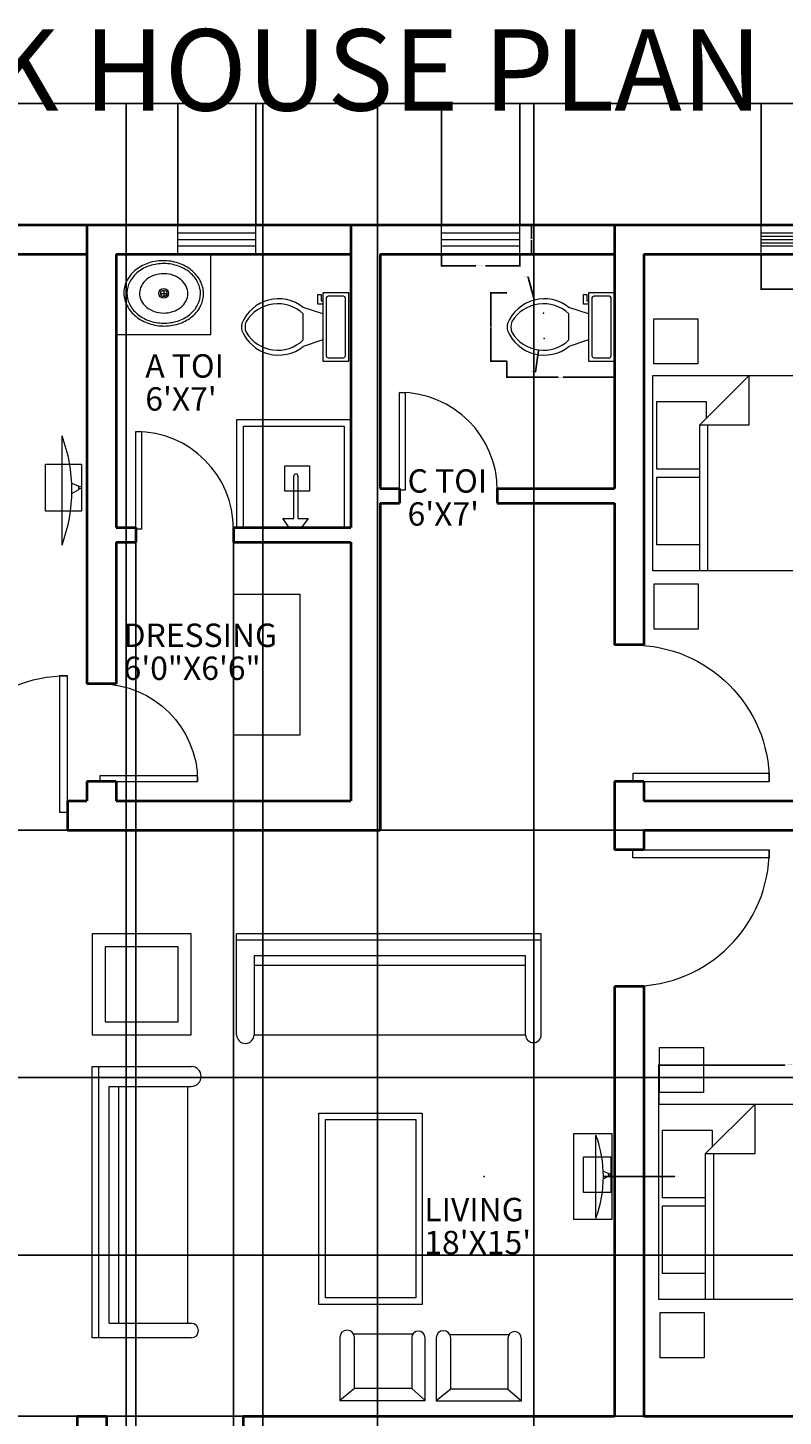
# Model space of a CAD drawing. Units: inches. Extents: x 12978 to 13669, y 46550 to 47327.
# Tile 4 of 5: x 13242 to 13474, y 46901 to 47327. Entities that reach past the tile are written whole.
import ezdxf

# ---------------------------------------------------------------- set-up
doc = ezdxf.new("R2010")
doc.units = ezdxf.units.IN
for name, color, linetype, lineweight in [('A-ANNO-DIMS', 2, 'Continuous', 18), ('A-ANNO-TITL', 7, 'Continuous', 35), ('A-AREA-IDEN', 1, 'Continuous', 18), ('A-EQPM', 8, 'Continuous', 18), ('A-FLOR-CASE', 8, 'Continuous', 20), ('A-FLOR-FIXT', 9, 'Continuous', 18), ('door', 4, 'Continuous', 20), ('furniture', 5, 'Continuous', 18), ('wall', 7, 'Continuous', 40), ('window', 1, 'Continuous', 18)]:
    doc.layers.add(name, color=color, linetype=linetype, lineweight=lineweight)
doc.styles.get("Standard").update_dxf_attribs({"font": 'arial.ttf'})
doc.dimstyles.get("Standard").update_dxf_attribs({"dimtxt": 0.18, "dimasz": 0.18, "dimexe": 0.18, "dimexo": 0.0625, "dimgap": 0.09, "dimtad": 0, "dimtih": 1, "dimtoh": 1, "dimdec": 4, "dimzin": 0, "dimdsep": 46, "dimtxsty": 'Standard', "dimcen": 0.09, "dimadec": 0, "dimazin": 0, "dimtfac": 1, "dimtdec": 4, "dimtofl": 0, "dimtmove": 0, "dimatfit": 3, "dimfxl": 1, "dimtolj": 1, "dimtzin": 0, "dimarcsym": 0})

# ---------------------------------------------------------------- blocks, each defined once
blk = doc.blocks.new('*U2')
for p, q in [((0, 0), (0, -100)), ((750, 0), (750, -100))]:
    blk.add_line(p, q)
blk.add_lwpolyline([(0, 0), (0, 750), (43.75, 750), (43.75, 0)], close=True)
blk.add_arc((0, 0), 750, 0, 90)
blk = doc.blocks.new('Bed - Queen')
for p, q in [((0, -80.00003), (0, 0)), ((0, 0), (59.99999, 0)), ((59.99999, 0), (59.99999, -80.00003)), ((7.99999, -1.2), (28.79998, -1.2)), ((7.99999, -14.4), (7.99999, -1.2)), ((28.79998, -1.2), (28.79998, -14.4)), ((31.19999, -1.2), (51.99999, -1.2)), ((31.19999, -14.4), (31.19999, -1.2)), ((51.99999, -1.2), (51.99999, -16.4)), ((0, -14.4), (44.8, -14.4)), ((44.8, -16.8), (0, -16.8)), ((59.99999, -29.6), (44.8, -14.4)), ((44.8, -14.4), (44.8, -29.6)), ((51.99999, -16.4), (46.79936, -16.4)), ((44.8, -29.6), (59.99999, -29.6)), ((59.99999, -80.00003), (0, -80.00003))]:
    blk.add_line(p, q)
blk = doc.blocks.new('Toilet - top')
for p, q in [((9.5, -6), (9.5, -2)), ((-10, -8.5), (-8, -8.5)), ((-10, -9.5), (-10, -8.5)), ((-8, -8.5), (-8, -8)), ((-7, -8), (-7, -9.5)), ((-4, -8), (-6, -14)), ((4, -8), (6, -14)), ((-7, -9.5), (-10, -9.5)), ((4, -14), (-4, -14))]:
    blk.add_line(p, q)
blk.add_lwpolyline([(10.5, -8), (10.5, 0), (-10.5, 0), (-10.5, -8)], close=True)
for points in [[(-9.5, -2), (-9.5, -6)], [(8.5, -1), (-8.5, -1)], [(-8.5, -7), (8.5, -7)]]:
    blk.add_lwpolyline(points)
for centre, radius, start, end in [((-8.62, -1.88), 0.884, 81.8699, 188.1301), ((8.62, -1.88), 0.884, 351.8699, 98.1301), ((-8.62, -6.12), 0.884, 171.8699, 278.1301), ((8.62, -6.12), 0.884, 261.8699, 8.1301), ((3.52, -21.58), 12.17, 141.4691, 247.9714), ((4.2, -21.82), 11.33, 136.3677, 238.9468), ((-3.52, -21.58), 12.17, 292.0284, 38.5307), ((-4.2, -21.82), 11.33, 301.053, 43.6321), ((0, -27.88), 4, 245.7318, 294.2682), ((0, -29), 4, 254.8605, 285.1395)]:
    blk.add_arc(centre, radius, start, end)
blk = doc.blocks.new('Sink - Oval top')
for p, q in [((-1, 0), (1, 0)), ((0, 1), (0, -1))]:
    blk.add_line(p, q)
for points in [[(-12.23, 0.39, 0.117634), (-11.46, -3.36, 0.104469), (-8.88, -6.8, 0.090016), (-5.08, -9.07, 0.08192), (-0.32, -10.02, 0.08192), (4.49, -9.38, 0.090016), (8.42, -7.36, 0.104469), (11.22, -4.09, 0.117634), (12.23, -0.39, 0.117634), (11.46, 3.36, 0.104469), (8.88, 6.8, 0.090016), (5.08, 9.07, 0.08192), (0.32, 10.02, 0.08192), (-4.49, 9.38, 0.090016), (-8.42, 7.36, 0.104469), (-11.22, 4.09, 0.117634)], [(-11.29, 0.16, 0.118622), (-10.52, -3.25, 0.104678), (-8.07, -6.36, 0.089562), (-4.54, -8.37, 0.081185), (-0.13, -9.15, 0.081185), (4.3, -8.49, 0.089562), (7.89, -6.58, 0.104678), (10.42, -3.55, 0.118622), (11.29, -0.16, 0.118622), (10.52, 3.25, 0.104678), (8.07, 6.36, 0.089562), (4.54, 8.37, 0.081185), (0.13, 9.15, 0.081185), (-4.3, 8.49, 0.089562), (-7.89, 6.58, 0.104678), (-10.42, 3.55, 0.118622)], [(-7.42, 0.08, 0.118283), (-6.91, -2.17, 0.104607), (-5.29, -4.21, 0.089718), (-2.97, -5.53, 0.081436), (-0.07, -6.04, 0.081436), (2.84, -5.59, 0.089718), (5.2, -4.33, 0.104607), (6.86, -2.32, 0.118283), (7.42, -0.08, 0.118283), (6.91, 2.17, 0.104607), (5.29, 4.21, 0.089718), (2.97, 5.53, 0.081436), (0.07, 6.04, 0.081436), (-2.84, 5.59, 0.089718), (-5.2, 4.33, 0.104607), (-6.86, 2.32, 0.118283)]]:
    blk.add_lwpolyline(points, format="xyb", close=True)
for radius in [1.5, 1]:
    blk.add_circle((0, 0), radius)
blk = doc.blocks.new('WINDOW-72')
for p, q in [((0, 0), (0, 9)), ((72, 0), (72, 9)), ((0, 6.5), (72, 6.5)), ((0, 5.5), (72, 5.5)), ((0, 4.5), (72, 4.5)), ((0, 3.5), (72, 3.5)), ((0, 2.5), (72, 2.5))]:
    blk.add_line(p, q)
blk = doc.blocks.new('WINDOW-24-BATH')
for p, q in [((0, 0), (0, 9)), ((24, 0), (24, 9)), ((0, 6.5), (24, 6.5)), ((0, 4.5), (24, 4.5)), ((0, 2.5), (24, 2.5))]:
    blk.add_line(p, q)
blk = doc.blocks.new('CHAIR-LOUNGE')
for p, q in [((21.6, 26.17), (2.34, 26.17)), ((17.92, 22.06), (21.6, 26.17)), ((21.6, 0), (21.6, 26.17)), ((1.14, 4.21), (1.14, 22.45)), ((2.34, 22.06), (17.92, 22.06)), ((17.92, 22.06), (17.92, 4.51)), ((17.92, 4.51), (2.25, 4.51)), ((17.92, 4.51), (21.6, 0)), ((2.25, 0), (21.6, 0))]:
    blk.add_line(p, q)
for centre, radius in [((2.34, 24.11), 2.05), ((2.25, 2.25), 2.25)]:
    blk.add_arc(centre, radius, 90, 270)
blk = doc.blocks.new('TV-FLATSCREEN')
for p, q in [((5.09, 0), (5.09, 33.56)), ((8.05, 19.02), (10.09, 18.18)), ((10.09, 18.18), (10.22, 17.01)), ((11.07, 17.34), (11.07, 18.07)), ((8.09, 15.82), (10.22, 17.01))]:
    blk.add_line(p, q)
blk.add_lwpolyline([(0, 24.86), (11.07, 24.86), (11.07, 10.37), (0, 10.37)], close=True)
blk.add_circle((10.63, 17.63), 0.418)
blk.add_arc((-40.12, 16.78), 48.22, 339.6348, 20.3652)
blk = doc.blocks.new('TABLE-BEDSIDE')
blk.add_lwpolyline([(0, 13.86), (13.51, 13.86), (13.51, 0), (0, 0)], close=True)
blk = doc.blocks.new('*D23')
at = {"layer": 'A-ANNO-DIMS', "color": 0, "lineweight": -2, "transparency": 16777216}
for p, q in [((13435.54, 46996.57), (13435.54, 47008.69)), ((13435.72, 47008.51), (13474.24, 47008.51)), ((13515.36, 47008.51), (13476.84, 47008.51)), ((13515.54, 46996.57), (13515.54, 47008.69))]:
    blk.add_line(p, q, dxfattribs=at)
at = {"layer": 'A-ANNO-DIMS', "color": 0, "transparency": 16777216}
for points in [[(13435.72, 47008.54), (13435.72, 47008.48), (13435.54, 47008.51)], [(13515.36, 47008.54), (13515.36, 47008.48), (13515.54, 47008.51)]]:
    blk.add_solid(points, dxfattribs=at)
at = {"layer": 'Defpoints', "color": 0, "transparency": 16777216}
for p in [(13435.54, 47008.51), (13435.54, 46996.51), (13515.54, 46996.51)]:
    blk.add_point(p, dxfattribs=at)
at = {"layer": 'A-ANNO-DIMS', "color": 0, "transparency": 16777216, "insert": (13475.54, 47008.51), "char_height": 0.18, "attachment_point": 5}
blk.add_mtext('\\A1;QUEEN BED 80 TYP.', dxfattribs=at)
blk = doc.blocks.new('*D33')
at = {"layer": 'A-ANNO-DIMS', "color": 0, "lineweight": -2, "transparency": 16777216}
for p, q in [((13466.96, 47257.57), (13466.96, 47246.65)), ((13538.96, 47257.57), (13538.96, 47246.65)), ((13467.14, 47246.83), (13501.84, 47246.83)), ((13538.78, 47246.83), (13504.08, 47246.83))]:
    blk.add_line(p, q, dxfattribs=at)
at = {"layer": 'A-ANNO-DIMS', "color": 0, "transparency": 16777216}
for points in [[(13467.14, 47246.86), (13467.14, 47246.8), (13466.96, 47246.83)], [(13538.78, 47246.86), (13538.78, 47246.8), (13538.96, 47246.83)]]:
    blk.add_solid(points, dxfattribs=at)
at = {"layer": 'Defpoints', "color": 0, "transparency": 16777216}
for p in [(13466.96, 47257.63), (13538.96, 47257.63), (13538.96, 47246.83)]:
    blk.add_point(p, dxfattribs=at)
at = {"layer": 'A-ANNO-DIMS', "color": 0, "transparency": 16777216, "insert": (13502.96, 47246.83), "char_height": 0.18, "attachment_point": 5}
blk.add_mtext('\\A1;WINDOW 72 TYP.', dxfattribs=at)
blk = doc.blocks.new('*D35')
at = {"layer": 'A-ANNO-DIMS', "color": 0, "lineweight": -2, "transparency": 16777216}
for p, q in [((13368.91, 47257.57), (13368.91, 47253.85)), ((13392.91, 47257.57), (13392.91, 47253.85)), ((13369.09, 47254.03), (13379.43, 47254.03)), ((13392.73, 47254.03), (13382.39, 47254.03))]:
    blk.add_line(p, q, dxfattribs=at)
at = {"layer": 'A-ANNO-DIMS', "color": 0, "transparency": 16777216}
for points in [[(13369.09, 47254.06), (13369.09, 47254), (13368.91, 47254.03)], [(13392.73, 47254.06), (13392.73, 47254), (13392.91, 47254.03)]]:
    blk.add_solid(points, dxfattribs=at)
at = {"layer": 'Defpoints', "color": 0, "transparency": 16777216}
for p in [(13368.91, 47257.63), (13392.91, 47257.63), (13392.91, 47254.03)]:
    blk.add_point(p, dxfattribs=at)
at = {"layer": 'A-ANNO-DIMS', "color": 0, "transparency": 16777216, "insert": (13380.91, 47254.03), "char_height": 0.18, "attachment_point": 5}
blk.add_mtext('\\A1;BATH WINDOW 24 TYP.', dxfattribs=at)
blk = doc.blocks.new('*D36')
at = {"layer": 'A-ANNO-DIMS', "color": 0, "lineweight": -2, "transparency": 16777216}
for p, q in [((13392.97, 47266.63), (13396.69, 47266.63)), ((13396.51, 47266.45), (13396.51, 47262.32)), ((13396.51, 47257.81), (13396.51, 47261.95)), ((13392.97, 47257.63), (13396.69, 47257.63))]:
    blk.add_line(p, q, dxfattribs=at)
at = {"layer": 'A-ANNO-DIMS', "color": 0, "transparency": 16777216}
for points in [[(13396.48, 47266.45), (13396.54, 47266.45), (13396.51, 47266.63)], [(13396.48, 47257.81), (13396.54, 47257.81), (13396.51, 47257.63)]]:
    blk.add_solid(points, dxfattribs=at)
at = {"layer": 'Defpoints', "color": 0, "transparency": 16777216}
for p in [(13392.91, 47266.63), (13396.51, 47266.63), (13392.91, 47257.63)]:
    blk.add_point(p, dxfattribs=at)
at = {"layer": 'A-ANNO-DIMS', "color": 0, "transparency": 16777216, "insert": (13396.51, 47262.13), "char_height": 0.18, "attachment_point": 5}
blk.add_mtext('\\A1;9 TYP.', dxfattribs=at)
blk = doc.blocks.new('*D37')
at = {"layer": 'A-ANNO-DIMS', "color": 0, "lineweight": -2, "transparency": 16777216}
for p, q in [((13388.96, 47224.7), (13388.96, 47219.62)), ((13422.01, 47224.7), (13422.01, 47219.62)), ((13389.14, 47219.8), (13404.71, 47219.8)), ((13421.83, 47219.8), (13406.26, 47219.8))]:
    blk.add_line(p, q, dxfattribs=at)
at = {"layer": 'A-ANNO-DIMS', "color": 0, "transparency": 16777216}
for points in [[(13389.14, 47219.83), (13389.14, 47219.77), (13388.96, 47219.8)], [(13421.83, 47219.83), (13421.83, 47219.77), (13422.01, 47219.8)]]:
    blk.add_solid(points, dxfattribs=at)
at = {"layer": 'Defpoints', "color": 0, "transparency": 16777216}
for p in [(13388.96, 47224.76), (13422.01, 47224.76), (13422.01, 47219.8)]:
    blk.add_point(p, dxfattribs=at)
at = {"layer": 'A-ANNO-DIMS', "color": 0, "transparency": 16777216, "insert": (13405.48, 47219.8), "char_height": 0.18, "attachment_point": 5}
blk.add_mtext('\\A1;WC 33 TYP.', dxfattribs=at)
blk = doc.blocks.new('*D38')
at = {"layer": 'A-ANNO-DIMS', "color": 0, "lineweight": -2, "transparency": 16777216}
for p, q in [((13388.9, 47245.76), (13383.82, 47245.76)), ((13384, 47245.58), (13384, 47235.44)), ((13384, 47224.94), (13384, 47235.08)), ((13388.9, 47224.76), (13383.82, 47224.76))]:
    blk.add_line(p, q, dxfattribs=at)
at = {"layer": 'A-ANNO-DIMS', "color": 0, "transparency": 16777216}
for points in [[(13383.97, 47245.58), (13384.03, 47245.58), (13384, 47245.76)], [(13383.97, 47224.94), (13384.03, 47224.94), (13384, 47224.76)]]:
    blk.add_solid(points, dxfattribs=at)
at = {"layer": 'Defpoints', "color": 0, "transparency": 16777216}
for p in [(13388.96, 47245.76), (13384, 47224.76), (13388.96, 47224.76)]:
    blk.add_point(p, dxfattribs=at)
at = {"layer": 'A-ANNO-DIMS', "color": 0, "transparency": 16777216, "insert": (13384, 47235.26), "char_height": 0.18, "attachment_point": 5}
blk.add_mtext('\\A1;21 TYP.', dxfattribs=at)
blk = doc.blocks.new('*D51')
at = {"layer": 'A-ANNO-DIMS', "color": 0, "lineweight": -2, "transparency": 16777216}
for p, q in [((13059.01, 47266.7), (13059.01, 47304.06)), ((13059.19, 47303.88), (13321.22, 47303.88)), ((13583.83, 47303.88), (13321.79, 47303.88)), ((13584.01, 47266.7), (13584.01, 47304.06))]:
    blk.add_line(p, q, dxfattribs=at)
at = {"layer": 'A-ANNO-DIMS', "color": 0, "transparency": 16777216}
for points in [[(13059.19, 47303.91), (13059.19, 47303.85), (13059.01, 47303.88)], [(13583.83, 47303.91), (13583.83, 47303.85), (13584.01, 47303.88)]]:
    blk.add_solid(points, dxfattribs=at)
at = {"layer": 'Defpoints', "color": 0, "transparency": 16777216}
for p in [(13584.01, 47303.88), (13059.01, 47266.63), (13584.01, 47266.63)]:
    blk.add_point(p, dxfattribs=at)
at = {"layer": 'A-ANNO-DIMS', "color": 0, "transparency": 16777216, "insert": (13321.51, 47303.88), "char_height": 0.18, "attachment_point": 5}
blk.add_mtext('\\A1;525', dxfattribs=at)
blk = doc.blocks.new('*D54')
at = {"layer": 'A-ANNO-DIMS', "color": 0, "lineweight": -2, "transparency": 16777216}
for p, q in [((13198.32, 47266.7), (13198.32, 47304.06)), ((13198.5, 47303.88), (13242.72, 47303.88)), ((13287.73, 47303.88), (13243.51, 47303.88)), ((13287.91, 47266.7), (13287.91, 47304.06))]:
    blk.add_line(p, q, dxfattribs=at)
at = {"layer": 'A-ANNO-DIMS', "color": 0, "transparency": 16777216}
for points in [[(13198.5, 47303.91), (13198.5, 47303.85), (13198.32, 47303.88)], [(13287.73, 47303.91), (13287.73, 47303.85), (13287.91, 47303.88)]]:
    blk.add_solid(points, dxfattribs=at)
at = {"layer": 'Defpoints', "color": 0, "transparency": 16777216}
for p in [(13287.91, 47303.88), (13198.32, 47266.63), (13287.91, 47266.63)]:
    blk.add_point(p, dxfattribs=at)
at = {"layer": 'A-ANNO-DIMS', "color": 0, "transparency": 16777216, "insert": (13243.12, 47303.88), "char_height": 0.18, "attachment_point": 5}
blk.add_mtext('\\A1;89.59', dxfattribs=at)
blk = doc.blocks.new('*D55')
at = {"layer": 'A-ANNO-DIMS', "color": 0, "lineweight": -2, "transparency": 16777216}
for p, q in [((13311.91, 47266.7), (13311.91, 47304.06)), ((13312.09, 47303.88), (13340.19, 47303.88)), ((13368.73, 47303.88), (13340.63, 47303.88)), ((13368.91, 47266.7), (13368.91, 47304.06))]:
    blk.add_line(p, q, dxfattribs=at)
at = {"layer": 'A-ANNO-DIMS', "color": 0, "transparency": 16777216}
for points in [[(13312.09, 47303.91), (13312.09, 47303.85), (13311.91, 47303.88)], [(13368.73, 47303.91), (13368.73, 47303.85), (13368.91, 47303.88)]]:
    blk.add_solid(points, dxfattribs=at)
at = {"layer": 'Defpoints', "color": 0, "transparency": 16777216}
for p in [(13368.91, 47303.88), (13311.91, 47266.63), (13368.91, 47266.63)]:
    blk.add_point(p, dxfattribs=at)
at = {"layer": 'A-ANNO-DIMS', "color": 0, "transparency": 16777216, "insert": (13340.41, 47303.88), "char_height": 0.18, "attachment_point": 5}
blk.add_mtext('\\A1;57', dxfattribs=at)
blk = doc.blocks.new('*D56')
at = {"layer": 'A-ANNO-DIMS', "color": 0, "lineweight": -2, "transparency": 16777216}
for p, q in [((13392.91, 47266.7), (13392.91, 47304.06)), ((13393.09, 47303.88), (13429.54, 47303.88)), ((13466.78, 47303.88), (13430.33, 47303.88)), ((13466.96, 47266.7), (13466.96, 47304.06))]:
    blk.add_line(p, q, dxfattribs=at)
at = {"layer": 'A-ANNO-DIMS', "color": 0, "transparency": 16777216}
for points in [[(13393.09, 47303.91), (13393.09, 47303.85), (13392.91, 47303.88)], [(13466.78, 47303.91), (13466.78, 47303.85), (13466.96, 47303.88)]]:
    blk.add_solid(points, dxfattribs=at)
at = {"layer": 'Defpoints', "color": 0, "transparency": 16777216}
for p in [(13466.96, 47303.88), (13392.91, 47266.63), (13466.96, 47266.63)]:
    blk.add_point(p, dxfattribs=at)
at = {"layer": 'A-ANNO-DIMS', "color": 0, "transparency": 16777216, "insert": (13429.93, 47303.88), "char_height": 0.18, "attachment_point": 5}
blk.add_mtext('\\A1;74.05', dxfattribs=at)
blk = doc.blocks.new('*D63')
at = {"layer": 'A-ANNO-DIMS', "color": 0, "lineweight": -2, "transparency": 16777216}
for p, q in [((13275.01, 47169.07), (13275.01, 46549.88)), ((13305.01, 47169.07), (13305.01, 46549.88)), ((13275.19, 46550.06), (13289.79, 46550.06)), ((13304.83, 46550.06), (13290.22, 46550.06))]:
    blk.add_line(p, q, dxfattribs=at)
at = {"layer": 'A-ANNO-DIMS', "color": 0, "transparency": 16777216}
for points in [[(13275.19, 46550.09), (13275.19, 46550.03), (13275.01, 46550.06)], [(13304.83, 46550.09), (13304.83, 46550.03), (13305.01, 46550.06)]]:
    blk.add_solid(points, dxfattribs=at)
at = {"layer": 'Defpoints', "color": 0, "transparency": 16777216}
for p in [(13275.01, 47169.13), (13305.01, 47169.13), (13305.01, 46550.06)]:
    blk.add_point(p, dxfattribs=at)
at = {"layer": 'A-ANNO-DIMS', "color": 0, "transparency": 16777216, "insert": (13290.01, 46550.06), "char_height": 0.18, "attachment_point": 5}
blk.add_mtext('\\A1;30', dxfattribs=at)
blk = doc.blocks.new('*D64')
at = {"layer": 'A-ANNO-DIMS', "color": 0, "lineweight": -2, "transparency": 16777216}
for p, q in [((13272.01, 46807.7), (13272.01, 47304.06)), ((13272.19, 47303.88), (13292.78, 47303.88)), ((13313.83, 47303.88), (13293.23, 47303.88)), ((13314.01, 46807.7), (13314.01, 47304.06))]:
    blk.add_line(p, q, dxfattribs=at)
at = {"layer": 'A-ANNO-DIMS', "color": 0, "transparency": 16777216}
for points in [[(13272.19, 47303.91), (13272.19, 47303.85), (13272.01, 47303.88)], [(13313.83, 47303.91), (13313.83, 47303.85), (13314.01, 47303.88)]]:
    blk.add_solid(points, dxfattribs=at)
at = {"layer": 'Defpoints', "color": 0, "transparency": 16777216}
for p in [(13314.01, 47303.88), (13272.01, 46807.63), (13314.01, 46807.63)]:
    blk.add_point(p, dxfattribs=at)
at = {"layer": 'A-ANNO-DIMS', "color": 0, "transparency": 16777216, "insert": (13293.01, 47303.88), "char_height": 0.18, "attachment_point": 5}
blk.add_mtext('\\A1;42', dxfattribs=at)
blk = doc.blocks.new('*D65')
at = {"layer": 'A-ANNO-DIMS', "color": 0, "lineweight": -2, "transparency": 16777216}
for p, q in [((13349.22, 46807.7), (13349.22, 47304.06)), ((13349.4, 47303.88), (13373, 47303.88)), ((13397.04, 47303.88), (13373.45, 47303.88)), ((13397.22, 46807.7), (13397.22, 47304.06))]:
    blk.add_line(p, q, dxfattribs=at)
at = {"layer": 'A-ANNO-DIMS', "color": 0, "transparency": 16777216}
for points in [[(13349.4, 47303.91), (13349.4, 47303.85), (13349.22, 47303.88)], [(13397.04, 47303.91), (13397.04, 47303.85), (13397.22, 47303.88)]]:
    blk.add_solid(points, dxfattribs=at)
at = {"layer": 'Defpoints', "color": 0, "transparency": 16777216}
for p in [(13397.22, 47303.88), (13349.22, 46807.63), (13397.22, 46807.63)]:
    blk.add_point(p, dxfattribs=at)
at = {"layer": 'A-ANNO-DIMS', "color": 0, "transparency": 16777216, "insert": (13373.22, 47303.88), "char_height": 0.18, "attachment_point": 5}
blk.add_mtext('\\A1;48', dxfattribs=at)
blk = doc.blocks.new('*D72')
at = {"layer": 'A-ANNO-DIMS', "color": 0, "lineweight": -2, "transparency": 16777216}
for p, q in [((13188.07, 46950.13), (13669.26, 46950.13)), ((13669.08, 46949.95), (13669.08, 46925.57)), ((13669.08, 46900.81), (13669.08, 46925.2)), ((13188.07, 46900.63), (13669.26, 46900.63))]:
    blk.add_line(p, q, dxfattribs=at)
at = {"layer": 'A-ANNO-DIMS', "color": 0, "transparency": 16777216}
for points in [[(13669.05, 46949.95), (13669.11, 46949.95), (13669.08, 46950.13)], [(13669.05, 46900.81), (13669.11, 46900.81), (13669.08, 46900.63)]]:
    blk.add_solid(points, dxfattribs=at)
at = {"layer": 'Defpoints', "color": 0, "transparency": 16777216}
for p in [(13188.01, 46950.13), (13669.08, 46950.13), (13188.01, 46900.63)]:
    blk.add_point(p, dxfattribs=at)
at = {"layer": 'A-ANNO-DIMS', "color": 0, "transparency": 16777216, "insert": (13669.08, 46925.38), "char_height": 0.18, "attachment_point": 5}
blk.add_mtext('\\A1;49.5', dxfattribs=at)
blk = doc.blocks.new('*D73')
at = {"layer": 'A-ANNO-DIMS', "color": 0, "lineweight": -2, "transparency": 16777216}
for p, q in [((13200.07, 47080.63), (13669.26, 47080.63)), ((13669.08, 47080.45), (13669.08, 47042.85)), ((13669.08, 47004.87), (13669.08, 47042.48)), ((13200.07, 47004.69), (13669.26, 47004.69))]:
    blk.add_line(p, q, dxfattribs=at)
at = {"layer": 'A-ANNO-DIMS', "color": 0, "transparency": 16777216}
for points in [[(13669.05, 47080.45), (13669.11, 47080.45), (13669.08, 47080.63)], [(13669.05, 47004.87), (13669.11, 47004.87), (13669.08, 47004.69)]]:
    blk.add_solid(points, dxfattribs=at)
at = {"layer": 'Defpoints', "color": 0, "transparency": 16777216}
for p in [(13200.01, 47080.63), (13669.08, 47080.63), (13200.01, 47004.69)]:
    blk.add_point(p, dxfattribs=at)
at = {"layer": 'A-ANNO-DIMS', "color": 0, "transparency": 16777216, "insert": (13669.08, 47042.66), "char_height": 0.18, "attachment_point": 5}
blk.add_mtext('\\A1;75.94', dxfattribs=at)
blk = doc.blocks.new('*D82')
at = {"layer": 'A-ANNO-DIMS', "color": 0, "lineweight": -2, "transparency": 16777216}
for p, q in [((13381.91, 46974.25), (13382.09, 46974.25)), ((13382, 46974.16), (13382, 46974.34)), ((13440.51, 46974.25), (13418.75, 46974.25))]:
    blk.add_line(p, q, dxfattribs=at)
at = {"layer": 'A-ANNO-DIMS', "color": 0, "transparency": 16777216}
blk.add_solid([(13418.75, 46974.28), (13418.75, 46974.22), (13418.57, 46974.25)], dxfattribs=at)
at = {"layer": 'Defpoints', "color": 0, "transparency": 16777216}
for p in [(13382, 46974.25), (13418.57, 46974.25)]:
    blk.add_point(p, dxfattribs=at)
at = {"layer": 'A-ANNO-DIMS', "color": 0, "transparency": 16777216, "insert": (13440.99, 46974.25), "char_height": 0.18, "attachment_point": 5}
blk.add_mtext('\\A1;R36.57', dxfattribs=at)
blk = doc.blocks.new('*D83')
at = {"layer": 'A-ANNO-DIMS', "color": 0, "lineweight": -2, "transparency": 16777216}
for p, q in [((13395.3, 47250.57), (13395.48, 47250.57)), ((13395.48, 47250.57), (13397.29, 47243.68)), ((13400.33, 47231.74), (13400.51, 47231.74)), ((13400.42, 47231.65), (13400.42, 47231.83))]:
    blk.add_line(p, q, dxfattribs=at)
at = {"layer": 'A-ANNO-DIMS', "color": 0, "transparency": 16777216}
blk.add_solid([(13397.32, 47243.69), (13397.26, 47243.67), (13397.33, 47243.51)], dxfattribs=at)
at = {"layer": 'Defpoints', "color": 0, "transparency": 16777216}
for p in [(13397.33, 47243.51), (13400.42, 47231.74)]:
    blk.add_point(p, dxfattribs=at)
at = {"layer": 'A-ANNO-DIMS', "color": 0, "transparency": 16777216, "insert": (13394.62, 47250.57), "char_height": 0.18, "attachment_point": 5}
blk.add_mtext('\\A1;4X R12.17', dxfattribs=at)
blk = doc.blocks.new('*D84')
at = {"layer": 'A-ANNO-DIMS', "color": 0, "lineweight": -2, "transparency": 16777216}
for p, q in [((13400.1, 47239.46), (13400.28, 47239.46)), ((13400.19, 47239.37), (13400.19, 47239.55)), ((13397.77, 47221.49), (13398.65, 47228.05)), ((13397.59, 47221.49), (13397.77, 47221.49))]:
    blk.add_line(p, q, dxfattribs=at)
at = {"layer": 'A-ANNO-DIMS', "color": 0, "transparency": 16777216}
blk.add_solid([(13398.62, 47228.06), (13398.68, 47228.05), (13398.68, 47228.23)], dxfattribs=at)
at = {"layer": 'Defpoints', "color": 0, "transparency": 16777216}
for p in [(13400.19, 47239.46), (13398.68, 47228.23)]:
    blk.add_point(p, dxfattribs=at)
at = {"layer": 'A-ANNO-DIMS', "color": 0, "transparency": 16777216, "insert": (13396.92, 47221.49), "char_height": 0.18, "attachment_point": 5}
blk.add_mtext('\\A1;4X R11.33', dxfattribs=at)

msp = doc.modelspace()

# ---------------------------------------------------------------- linework, layer by layer
at = {"layer": 'A-EQPM'}
for p, q in [((13416.2806, 46961.5191), (13416.2806, 46986.9724)), ((13418.5269, 46975.9472), (13420.0729, 46975.3091)), ((13418.5592, 46973.5193), (13420.1715, 46974.4229)), ((13420.0729, 46975.3091), (13420.1715, 46974.4229)), ((13420.8201, 46974.6677), (13420.8201, 46975.2251))]:
    msp.add_line(p, q, dxfattribs=at)
for points in [[(13409.5043, 46987.4664), (13421.1135, 46987.4664), (13421.1135, 46961.1051), (13409.5043, 46961.1051)], [(13412.4229, 46980.3713), (13420.8201, 46980.3713), (13420.8201, 46969.3833), (13412.4229, 46969.3833)]]:
    msp.add_lwpolyline(points, close=True, dxfattribs=at)
msp.add_circle((13420.4851, 46974.8881), 0.3173, dxfattribs=at)
msp.add_arc((13381.9959, 46974.2458), 36.5706, 339.634793, 20.365207, dxfattribs=at)
at = {"layer": 'A-FLOR-CASE'}
for p, q in [((13298.0485, 47232.9572), (13298.0485, 47257.6345)), ((13269.005, 47232.9572), (13298.0485, 47232.9572)), ((13305.005, 47169.1345), (13305.005, 47153.1868)), ((13305.005, 47153.1868), (13325.3347, 47153.1868)), ((13325.3347, 47153.1868), (13325.3347, 47109.8458)), ((13325.3347, 47109.8458), (13305.005, 47109.8458)), ((13305.005, 47109.8458), (13305.005, 47089.6345))]:
    msp.add_line(p, q, dxfattribs=at)
at = {"layer": 'A-FLOR-FIXT'}
for p, q in [((13308.0318, 47173.6345), (13308.0318, 47204.7951)), ((13308.0318, 47204.7951), (13339.005, 47204.7951)), ((13339.005, 47204.7951), (13339.005, 47173.6345)), ((13323.5184, 47176.4476), (13323.5184, 47189.4346)), ((13324.8026, 47189.4346), (13324.8026, 47176.4476)), ((13322.0938, 47173.6345), (13320.1891, 47176.4476)), ((13320.1891, 47176.4476), (13323.5184, 47176.4476)), ((13324.8026, 47176.4476), (13327.8799, 47176.4476)), ((13327.8799, 47176.4476), (13325.9151, 47173.6345))]:
    msp.add_line(p, q, dxfattribs=at)
for points in [[(13341.005, 47173.6345), (13306.0318, 47173.6345), (13306.0318, 47206.7951), (13341.005, 47206.7951)], [(13320.7473, 47192.5762), (13328.3481, 47192.5762), (13328.3481, 47184.7994), (13320.7473, 47184.7994)]]:
    msp.add_lwpolyline(points, close=True, dxfattribs=at)
msp.add_arc((13324.1605, 47189.4346), 0.6421, 0, 180, dxfattribs=at)
at = {"layer": 'furniture'}
for p, q in [((13261.6156, 47048.8336), (13261.6156, 47017.8148)), ((13292.0247, 47048.8336), (13261.6156, 47048.8336)), ((13292.0247, 47017.8148), (13292.0247, 47048.8336)), ((13399.5076, 47048.8336), (13305.975, 47048.8336)), ((13305.975, 47017.8148), (13305.975, 47048.8336)), ((13399.5076, 47046.8336), (13305.975, 47046.8336)), ((13399.5076, 47017.8148), (13399.5076, 47048.8336)), ((13288.0247, 47044.8336), (13265.6156, 47044.8336)), ((13265.6156, 47044.8336), (13265.6156, 47021.8148)), ((13288.0247, 47021.8148), (13288.0247, 47044.8336)), ((13394.6633, 47042.1071), (13311.3365, 47042.1071)), ((13311.3365, 47042.1071), (13311.3365, 47017.8148)), ((13394.6633, 47017.8148), (13394.6633, 47042.1071)), ((13394.6633, 47039.1071), (13311.3365, 47039.1071)), ((13265.6156, 47021.8148), (13288.0247, 47021.8148)), ((13261.6156, 47017.8148), (13292.0247, 47017.8148)), ((13311.3365, 47017.8148), (13394.6633, 47017.8148)), ((13261.6156, 47008.0587), (13292.0247, 47008.0587)), ((13261.6156, 46924.6956), (13261.6156, 47008.0587)), ((13263.6156, 46924.6956), (13263.6156, 47008.0587)), ((13266.8155, 47001.9588), (13292.0247, 47001.9588)), ((13266.8155, 46929.2009), (13266.8155, 47001.9588)), ((13269.8155, 46929.2009), (13269.8155, 47001.9588)), ((13291.0077, 46929.2009), (13291.0077, 47001.9588)), ((13266.8155, 46929.2009), (13292.0247, 46929.2009)), ((13292.0247, 46924.6956), (13261.6156, 46924.6956))]:
    msp.add_line(p, q, dxfattribs=at)
for points in [[(13331.2443, 46993.7758), (13362.9475, 46993.7758), (13362.9475, 46934.9694), (13331.2443, 46934.9694)], [(13333.2443, 46991.7758), (13360.9475, 46991.7758), (13360.9475, 46936.9694), (13333.2443, 46936.9694)]]:
    msp.add_lwpolyline(points, close=True, dxfattribs=at)
for centre, radius, start, end in [((13308.6557, 47017.8148), 2.6807, 180, 0), ((13397.0855, 47017.8148), 2.4221, 180, 0), ((13292.0247, 47005.0088), 3.0499, 270, 90), ((13292.0247, 46926.9483), 2.2526, 270, 90)]:
    msp.add_arc(centre, radius, start, end, dxfattribs=at)
at = {"layer": 'wall'}
for p, q in [((13059.005, 47266.6345), (13584.005, 47266.6345)), ((13260.005, 47266.6345), (13260.005, 47125.6345)), ((13341.005, 47266.6345), (13341.005, 47173.6345)), ((13422.005, 47266.6345), (13422.005, 47185.6345)), ((13068.005, 47257.6345), (13260.005, 47257.6345)), ((13269.005, 47257.6345), (13269.005, 47173.6345)), ((13269.005, 47257.6345), (13341.005, 47257.6345)), ((13350.005, 47257.6345), (13350.005, 47185.6345)), ((13350.005, 47257.6345), (13422.005, 47257.6345)), ((13431.005, 47257.6345), (13431.005, 47137.6345)), ((13431.005, 47257.6345), (13575.005, 47257.6345)), ((13350.005, 47185.6345), (13356.005, 47185.6345)), ((13356.005, 47185.6345), (13356.005, 47181.1345)), ((13386.005, 47185.6345), (13386.005, 47181.1345)), ((13386.005, 47185.6345), (13422.005, 47185.6345)), ((13350.005, 47181.1345), (13356.005, 47181.1345)), ((13350.005, 47181.1345), (13350.005, 47080.6345)), ((13386.005, 47181.1345), (13422.005, 47181.1345)), ((13422.005, 47181.1345), (13422.005, 47137.6345)), ((13269.005, 47173.6345), (13275.005, 47173.6345)), ((13275.005, 47173.6345), (13275.005, 47169.1345)), ((13305.005, 47173.6345), (13305.005, 47169.1345)), ((13305.005, 47173.6345), (13341.005, 47173.6345)), ((13269.005, 47169.1345), (13275.005, 47169.1345)), ((13269.005, 47169.1345), (13269.005, 47125.6345)), ((13305.005, 47169.1345), (13341.005, 47169.1345)), ((13341.005, 47169.1345), (13341.005, 47089.6345)), ((13431.005, 47137.6345), (13422.005, 47137.6345)), ((13269.005, 47125.6345), (13260.005, 47125.6345)), ((13269.005, 47095.6345), (13260.005, 47095.6345)), ((13260.005, 47095.6345), (13260.005, 47089.6345)), ((13269.005, 47095.6345), (13269.005, 47089.6345)), ((13431.005, 47095.6345), (13422.005, 47095.6345)), ((13422.005, 47095.6345), (13422.005, 47089.6345)), ((13431.005, 47095.6345), (13431.005, 47089.6345)), ((13254.005, 47089.6345), (13254.005, 47080.6345)), ((13254.005, 47089.6345), (13260.005, 47089.6345)), ((13269.005, 47089.6345), (13341.005, 47089.6345)), ((13422.005, 47089.6345), (13422.005, 47074.6345)), ((13431.005, 47089.6345), (13575.005, 47089.6345)), ((13254.005, 47080.6345), (13350.005, 47080.6345)), ((13431.005, 47080.6345), (13431.005, 47074.6345)), ((13431.005, 47080.6345), (13575.005, 47080.6345)), ((13431.005, 47074.6345), (13422.005, 47074.6345)), ((13431.005, 47032.6345), (13422.005, 47032.6345)), ((13422.005, 47032.6345), (13422.005, 46900.6345)), ((13431.005, 47032.6345), (13431.005, 46900.6345)), ((13257.005, 46900.6345), (13257.005, 46660.6345)), ((13257.005, 46900.6345), (13266.005, 46900.6345)), ((13266.005, 46900.6345), (13266.005, 46807.6345)), ((13308.005, 46900.6345), (13422.005, 46900.6345)), ((13308.005, 46900.6345), (13308.005, 46891.6345)), ((13431.005, 46900.6345), (13575.005, 46900.6345))]:
    msp.add_line(p, q, dxfattribs=at)

# ---------------------------------------------------------------- block references
at = {"layer": 'A-EQPM'}
msp.add_blockref('TV-FLATSCREEN', (13247.2754, 47168.2685), dxfattribs=at)
at = {"layer": 'A-FLOR-FIXT'}
msp.add_blockref('Sink - Oval top', (13283.5811, 47245.5756), dxfattribs=at)
at = {"layer": 'A-FLOR-FIXT', "rotation": 270}
for p in [(13340.4253, 47235.2578), (13422.005, 47235.2578)]:
    msp.add_blockref('Toilet - top', p, dxfattribs=at)
at = {"layer": 'door'}
for p, xscale, yscale, zscale in [((13356.005, 47185.1345), 0.0400000000000011, 0.0400000000000011, 0.0400000000000011), ((13275.005, 47173.1345), 0.0400000000000011, 0.0400000000000011, 0.0400000000000011), ((13254.005, 47086.222), -0.0558759688399716, 0.0558759688399716, 0.0558759688399716)]:
    msp.add_blockref('*U2', p, dxfattribs=dict(at, xscale=xscale, yscale=yscale, zscale=zscale))
at = {"layer": 'door', "rotation": 270}
for p, xscale, yscale, zscale in [((13427.5926, 47095.6345), -0.0558759688399716, 0.0558759688399716, 0.0558759688399716), ((13264.005, 47095.6345), -0.0400000000000011, 0.0400000000000011, 0.0400000000000011), ((13427.5926, 47074.6345), 0.0558759688399716, 0.0558759688399716, 0.0558759688399716)]:
    msp.add_blockref('*U2', p, dxfattribs=dict(at, xscale=xscale, yscale=yscale, zscale=zscale))
at = {"layer": 'furniture'}
for p in [(13434.0152, 47223.9278), (13434.1875, 47142.4435), (13435.8043, 47000.0784), (13435.9766, 46918.5942)]:
    msp.add_blockref('TABLE-BEDSIDE', p, dxfattribs=at)
for name, p, rotation in [('Bed - Queen', (13433.7494, 47160.3603), 90), ('Bed - Queen', (13435.5385, 46936.511), 90), ('CHAIR-LOUNGE', (13337.649, 46927.0925), 270.0000000000255), ('CHAIR-LOUNGE', (13367.208, 46926.9167), 270.0000000000255)]:
    msp.add_blockref(name, p, dxfattribs=dict(at, rotation=rotation))
at = {"layer": 'window'}
for name, p in [('WINDOW-24-BATH', (13287.9094, 47257.6345)), ('WINDOW-24-BATH', (13368.9094, 47257.6345)), ('WINDOW-72', (13466.959, 47257.6345))]:
    msp.add_blockref(name, p, dxfattribs=at)

# ---------------------------------------------------------------- texts
at = {"layer": 'A-ANNO-TITL'}
msp.add_text('3BHK HOUSE PLAN', height=25.000014, dxfattribs=at).set_placement((13163.1704, 47301.722))
at = {"layer": 'A-AREA-IDEN'}
for s, p in [('A TOI', (13277.9298, 47219.6907)), ("6'X7'", (13277.9298, 47209.5522)), ('C TOI', (13358.4481, 47184.3521)), ("6'X7'", (13358.4481, 47174.2136)), ('DRESSING', (13271.2655, 47136.9567)), ('6\'0"X6\'6"', (13271.2655, 47126.8182)), ('LIVING', (13363.5852, 46960.5447)), ("18'X15'", (13363.5852, 46950.4062))]:
    msp.add_text(s, height=7.17855, dxfattribs=at).set_placement(p)

# ---------------------------------------------------------------- dimensions: what is measured, and where the dimension line sits
at = {"layer": 'A-ANNO-DIMS'}
for base, p1, p2, override, picture, middle in [((13584.005, 47303.8845), (13059.005, 47266.6345), (13584.005, 47266.6345), {"dimdec": 0, "dimlfac": 1, "dimrnd": 0, "dimzin": 0, "dimdsep": 46, "dimlunit": 2}, '*D51', (13321.505, 47303.8845)), ((13287.9094, 47303.8845), (13198.3221, 47266.6345), (13287.9094, 47266.6345), {"dimdec": 2, "dimlfac": 1, "dimrnd": 0, "dimzin": 0, "dimdsep": 46, "dimlunit": 2}, '*D54', (13243.1158, 47303.8845)), ((13314.005, 47303.8845), (13272.005, 46807.6345), (13314.005, 46807.6345), {"dimdec": 0, "dimlfac": 1, "dimrnd": 0, "dimzin": 0, "dimdsep": 46, "dimlunit": 2}, '*D64', (13293.005, 47303.8845)), ((13368.9094, 47303.8845), (13311.9094, 47266.6345), (13368.9094, 47266.6345), {"dimdec": 0, "dimlfac": 1, "dimrnd": 0, "dimzin": 0, "dimdsep": 46, "dimlunit": 2}, '*D55', (13340.4094, 47303.8845)), ((13397.2243, 47303.8845), (13349.2243, 46807.6345), (13397.2243, 46807.6345), {"dimdec": 0, "dimlfac": 1, "dimrnd": 0, "dimzin": 0, "dimdsep": 46, "dimlunit": 2}, '*D65', (13373.2243, 47303.8845)), ((13466.959, 47303.8845), (13392.9094, 47266.6345), (13466.959, 47266.6345), {"dimdec": 2, "dimlfac": 1, "dimrnd": 0, "dimzin": 0, "dimdsep": 46, "dimlunit": 2}, '*D56', (13429.9342, 47303.8845)), ((13305.005, 46550.0575), (13275.005, 47169.1345), (13305.005, 47169.1345), {"dimdec": 0, "dimlfac": 1, "dimrnd": 0, "dimzin": 0, "dimdsep": 46, "dimlunit": 2}, '*D63', (13290.005, 46550.0575))]:
    dim = msp.add_linear_dim(base=base, p1=p1, p2=p2, dimstyle='Standard', override=override, dxfattribs=at)
    dim.commit()
    dim.dimension.update_dxf_attribs({"geometry": picture, "text_midpoint": middle})
for base, p1, p2, angle, text, picture, middle in [((13396.5094, 47266.6345), (13392.9094, 47257.6345), (13392.9094, 47266.6345), 90, '<> TYP.', '*D36', (13396.5094, 47262.1345)), ((13384.0018, 47224.7578), (13388.9588, 47245.7578), (13388.9588, 47224.7578), 270, '<> TYP.', '*D38', (13384.0018, 47235.2578)), ((13435.5385, 47008.511), (13515.5385, 46996.511), (13435.5385, 46996.511), 180, 'QUEEN BED <> TYP.', '*D23', (13475.5385, 47008.511))]:
    dim = msp.add_linear_dim(base=base, p1=p1, p2=p2, angle=angle, text=text, dimstyle='Standard', override={"dimdec": 0, "dimlfac": 1, "dimrnd": 0, "dimzin": 0, "dimdsep": 46, "dimlunit": 2}, dxfattribs=at)
    dim.commit()
    dim.dimension.update_dxf_attribs({"geometry": picture, "text_midpoint": middle})
for base, p1, p2, text, picture, middle in [((13392.9094, 47254.0345), (13368.9094, 47257.6345), (13392.9094, 47257.6345), 'BATH WINDOW <> TYP.', '*D35', (13380.9094, 47254.0345)), ((13538.959, 47246.8345), (13466.959, 47257.6345), (13538.959, 47257.6345), 'WINDOW <> TYP.', '*D33', (13502.959, 47246.8345)), ((13422.005, 47219.8009), (13388.9588, 47224.7578), (13422.005, 47224.7578), 'WC <> TYP.', '*D37', (13405.4819, 47219.8009))]:
    dim = msp.add_linear_dim(base=base, p1=p1, p2=p2, text=text, dimstyle='Standard', override={"dimdec": 0, "dimlfac": 1, "dimrnd": 0, "dimzin": 0, "dimdsep": 46, "dimlunit": 2}, dxfattribs=at)
    dim.commit()
    dim.dimension.update_dxf_attribs({"geometry": picture, "text_midpoint": middle})
for center, mpoint, picture, middle in [((13400.4245, 47231.7383), (13397.3321, 47243.5078), '*D83', (13394.6197, 47250.5695)), ((13400.1876, 47239.4577), (13398.6779, 47228.2296), '*D84', (13396.9153, 47221.4927))]:
    dim = msp.add_radius_dim(center=center, mpoint=mpoint, text='4X <>', dimstyle='Standard', override={"dimdec": 2, "dimlfac": 1, "dimrnd": 0, "dimzin": 0, "dimdsep": 46, "dimlunit": 2}, dxfattribs=at)
    dim.commit()
    dim.dimension.update_dxf_attribs({"geometry": picture, "text_midpoint": middle, "dimtype": 164})
for base, p1, p2, override, picture, middle in [((13669.0793, 47080.6345), (13200.005, 47004.6918), (13200.005, 47080.6345), {"dimdec": 2, "dimlfac": 1, "dimrnd": 0, "dimzin": 0, "dimdsep": 46, "dimlunit": 2}, '*D73', (13669.0793, 47042.6631)), ((13669.0793, 46950.1345), (13188.005, 46900.6345), (13188.005, 46950.1345), {"dimdec": 1, "dimlfac": 1, "dimrnd": 0, "dimzin": 0, "dimdsep": 46, "dimlunit": 2}, '*D72', (13669.0793, 46925.3845))]:
    dim = msp.add_linear_dim(base=base, p1=p1, p2=p2, angle=90, dimstyle='Standard', override=override, dxfattribs=at)
    dim.commit()
    dim.dimension.update_dxf_attribs({"geometry": picture, "text_midpoint": middle})
dim = msp.add_radius_dim(center=(13381.9959, 46974.2458), mpoint=(13418.5665, 46974.246), dimstyle='Standard', override={"dimdec": 2, "dimlfac": 1, "dimrnd": 0, "dimzin": 0, "dimdsep": 46, "dimlunit": 2}, dxfattribs=at)
dim.commit()
dim.dimension.update_dxf_attribs({"geometry": '*D82', "text_midpoint": (13440.5088, 46974.2461), "dimtype": 164})

doc.saveas('drawing.dxf')
